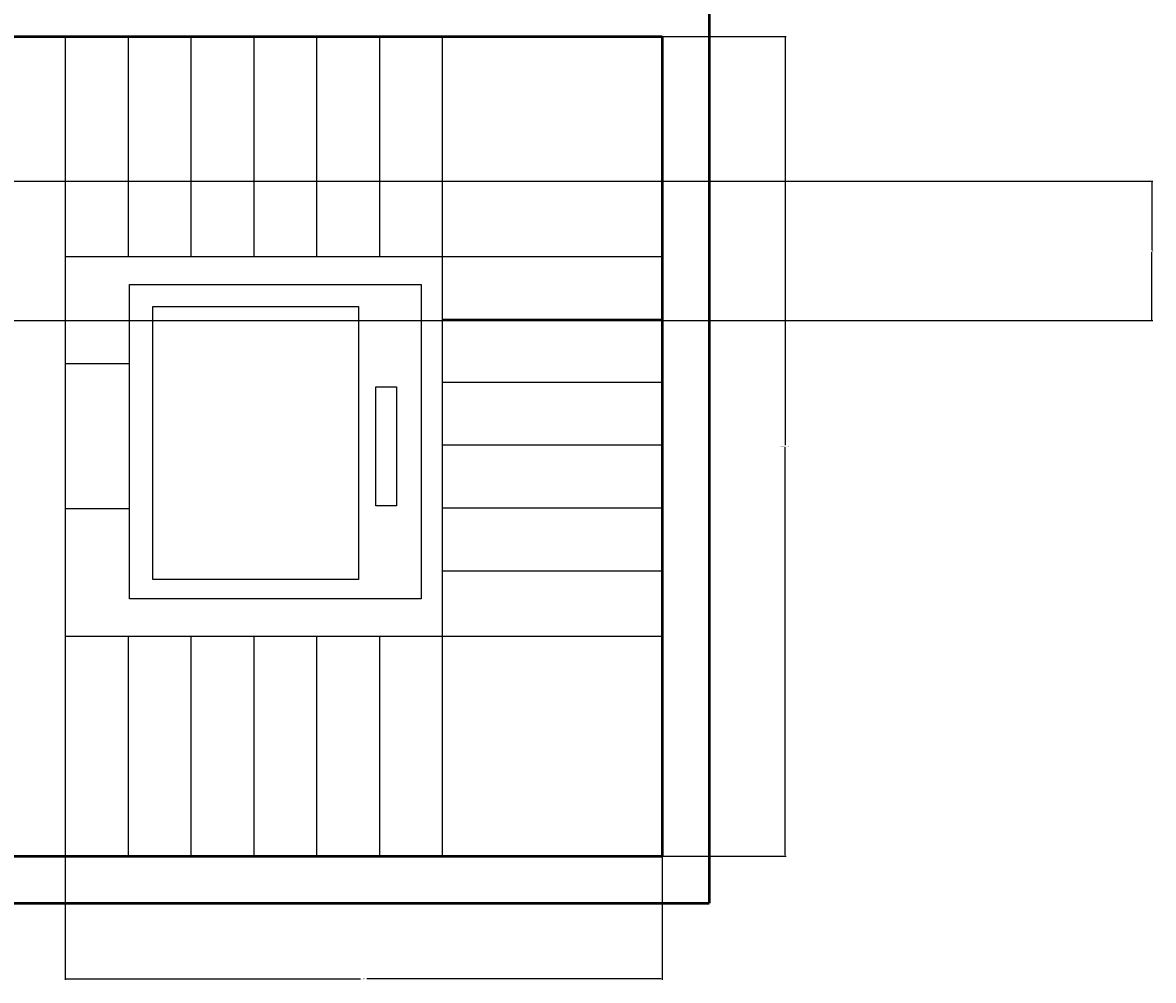
# Model space of a CAD drawing. Units: inches. Extents: x 7359 to 7979, y 33027 to 34263.
# Tile 30 of 32: x 7753 to 7969, y 33750 to 33933. Entities that reach past the tile are written whole.
import ezdxf

# ---------------------------------------------------------------- set-up
doc = ezdxf.new("R2010")
doc.units = ezdxf.units.IN
for name, color, linetype, lineweight in [('A-ANNO-DIMS', 2, 'Continuous', 18), ('A-CONV', 6, 'Continuous', 25), ('A-FLOR-STRS', 7, 'Continuous', 25), ('A-WALL', 7, 'Continuous', 50)]:
    doc.layers.add(name, color=color, linetype=linetype, lineweight=lineweight)
doc.styles.get("Standard").update_dxf_attribs({"font": 'arial.ttf'})
doc.dimstyles.get("Standard").update_dxf_attribs({"dimtxt": 0.18, "dimasz": 0.18, "dimexe": 0.18, "dimexo": 0.0625, "dimgap": 0.09, "dimtad": 0, "dimtih": 1, "dimtoh": 1, "dimdec": 4, "dimzin": 0, "dimdsep": 46, "dimtxsty": 'Standard', "dimcen": 0.09, "dimadec": 0, "dimazin": 0, "dimtfac": 1, "dimtdec": 4, "dimtofl": 0, "dimtmove": 0, "dimatfit": 3, "dimfxl": 1, "dimtolj": 1, "dimtzin": 0, "dimarcsym": 0})

# ---------------------------------------------------------------- blocks, each defined once
blk = doc.blocks.new('STAIR-THREE-FLIGHT')
for p, q in [((0, 156.5), (0, 114.5)), ((12, 156.5), (12, 114.5)), ((24, 156.5), (24, 114.5)), ((36, 156.5), (36, 114.5)), ((48, 156.5), (48, 114.5)), ((60, 156.5), (60, 114.5)), ((72, 156.5), (72, 0)), ((0, 114.5), (114, 114.5)), ((0, 114.5), (0, 42)), ((72, 102.5), (114, 102.5)), ((72, 90.5), (114, 90.5)), ((72, 78.5), (114, 78.5)), ((72, 66.5), (114, 66.5)), ((72, 54.5), (114, 54.5)), ((0, 42), (114, 42)), ((0, 42), (0, 0)), ((12, 42), (12, 0)), ((24, 42), (24, 0)), ((36, 42), (36, 0)), ((48, 42), (48, 0)), ((60, 42), (60, 0))]:
    blk.add_line(p, q)
blk = doc.blocks.new('LIFT-PLAN')
for p, q in [((0, 44.9), (12.25, 44.9)), ((0, 17.24), (12.25, 17.24))]:
    blk.add_line(p, q)
for points in [[(12.25, 60.03), (67.98, 60.03), (67.98, 0), (12.25, 0)], [(16.72, 55.81), (56.03, 55.81), (56.03, 3.68), (16.72, 3.68)], [(59.32, 40.45), (63.26, 40.45), (63.26, 17.73), (59.32, 17.73)]]:
    blk.add_lwpolyline(points, close=True)
blk = doc.blocks.new('*D50')
at = {"layer": 'A-ANNO-DIMS', "color": 0, "lineweight": -2, "transparency": 16777216}
for p, q in [((7875.05, 33930.33), (7898.65, 33930.33)), ((7898.47, 33930.15), (7898.47, 33852.27)), ((7898.47, 33774.01), (7898.47, 33851.9)), ((7875.05, 33773.83), (7898.65, 33773.83))]:
    blk.add_line(p, q, dxfattribs=at)
at = {"layer": 'A-ANNO-DIMS', "color": 0, "transparency": 16777216}
for points in [[(7898.44, 33930.15), (7898.5, 33930.15), (7898.47, 33930.33)], [(7898.44, 33774.01), (7898.5, 33774.01), (7898.47, 33773.83)]]:
    blk.add_solid(points, dxfattribs=at)
at = {"layer": 'Defpoints', "color": 0, "transparency": 16777216}
for p in [(7874.99, 33930.33), (7898.47, 33930.33), (7874.99, 33773.83)]:
    blk.add_point(p, dxfattribs=at)
at = {"layer": 'A-ANNO-DIMS', "color": 0, "transparency": 16777216, "insert": (7898.47, 33852.08), "char_height": 0.18, "attachment_point": 5}
blk.add_mtext('\\A1;STAIR 157 TYP.', dxfattribs=at)
blk = doc.blocks.new('*D51')
at = {"layer": 'A-ANNO-DIMS', "color": 0, "lineweight": -2, "transparency": 16777216}
for p, q in [((7760.99, 33773.77), (7760.99, 33750.18)), ((7874.99, 33773.77), (7874.99, 33750.18)), ((7761.17, 33750.36), (7817.4, 33750.36)), ((7874.81, 33750.36), (7818.58, 33750.36))]:
    blk.add_line(p, q, dxfattribs=at)
at = {"layer": 'A-ANNO-DIMS', "color": 0, "transparency": 16777216}
for points in [[(7761.17, 33750.39), (7761.17, 33750.33), (7760.99, 33750.36)], [(7874.81, 33750.39), (7874.81, 33750.33), (7874.99, 33750.36)]]:
    blk.add_solid(points, dxfattribs=at)
at = {"layer": 'Defpoints', "color": 0, "transparency": 16777216}
for p in [(7760.99, 33773.83), (7874.99, 33773.83), (7874.99, 33750.36)]:
    blk.add_point(p, dxfattribs=at)
at = {"layer": 'A-ANNO-DIMS', "color": 0, "transparency": 16777216, "insert": (7817.99, 33750.36), "char_height": 0.18, "attachment_point": 5}
blk.add_mtext('\\A1;114 TYP.', dxfattribs=at)
blk = doc.blocks.new('*D82')
at = {"layer": 'A-ANNO-DIMS', "color": 0, "lineweight": -2, "transparency": 16777216}
for p, q in [((7689.55, 33902.73), (7968.68, 33902.73)), ((7968.5, 33902.55), (7968.5, 33889.59)), ((7968.5, 33876.26), (7968.5, 33889.23)), ((7689.55, 33876.08), (7968.68, 33876.08))]:
    blk.add_line(p, q, dxfattribs=at)
at = {"layer": 'A-ANNO-DIMS', "color": 0, "transparency": 16777216}
for points in [[(7968.47, 33902.55), (7968.53, 33902.55), (7968.5, 33902.73)], [(7968.47, 33876.26), (7968.53, 33876.26), (7968.5, 33876.08)]]:
    blk.add_solid(points, dxfattribs=at)
at = {"layer": 'Defpoints', "color": 0, "transparency": 16777216}
for p in [(7689.49, 33902.73), (7968.5, 33902.73), (7689.49, 33876.08)]:
    blk.add_point(p, dxfattribs=at)
at = {"layer": 'A-ANNO-DIMS', "color": 0, "transparency": 16777216, "insert": (7968.5, 33889.41), "char_height": 0.18, "attachment_point": 5}
blk.add_mtext('\\A1;26.65', dxfattribs=at)

msp = doc.modelspace()

# ---------------------------------------------------------------- linework, layer by layer
at = {"layer": 'A-WALL'}
for p, q in [((7883.9915, 34233.3339), (7883.9915, 33764.8339)), ((7698.4915, 33930.3339), (7874.9915, 33930.3339)), ((7874.9915, 33930.3339), (7874.9915, 33773.8339)), ((7698.4915, 33773.8339), (7874.9915, 33773.8339)), ((7458.5915, 33764.8339), (7883.9915, 33764.8339))]:
    msp.add_line(p, q, dxfattribs=at)

# ---------------------------------------------------------------- block references
at = {"layer": 'A-CONV'}
msp.add_blockref('LIFT-PLAN', (7760.991, 33822.985), dxfattribs=at)
at = {"layer": 'A-FLOR-STRS'}
msp.add_blockref('STAIR-THREE-FLIGHT', (7760.991, 33773.834), dxfattribs=at)

# ---------------------------------------------------------------- dimensions: what is measured, and where the dimension line sits
at = {"layer": 'A-ANNO-DIMS'}
dim = msp.add_linear_dim(base=(7898.4664840368, 33930.3339283577), p1=(7874.9914840368, 33773.8339283577), p2=(7874.9914840368, 33930.3339283577), angle=90, text='STAIR <> TYP.', dimstyle='Standard', override={"dimdec": 0, "dimlfac": 1, "dimrnd": 0, "dimzin": 0, "dimdsep": 46, "dimlunit": 2}, dxfattribs=at)
dim.commit()
dim.dimension.update_dxf_attribs({"geometry": '*D50', "text_midpoint": (7898.4664840368, 33852.0839283577)})
dim = msp.add_linear_dim(base=(7968.502, 33902.7339), p1=(7689.4915, 33876.0839), p2=(7689.4915, 33902.7339), angle=90, dimstyle='Standard', override={"dimdec": 2, "dimlfac": 1, "dimrnd": 0, "dimzin": 0, "dimdsep": 46, "dimlunit": 2}, dxfattribs=at)
dim.commit()
dim.dimension.update_dxf_attribs({"geometry": '*D82', "text_midpoint": (7968.502, 33889.4089)})
dim = msp.add_linear_dim(base=(7874.9915, 33750.3589), p1=(7760.9915, 33773.8339), p2=(7874.9915, 33773.8339), text='<> TYP.', dimstyle='Standard', override={"dimdec": 0, "dimlfac": 1, "dimrnd": 0, "dimzin": 0, "dimdsep": 46, "dimlunit": 2}, dxfattribs=at)
dim.commit()
dim.dimension.update_dxf_attribs({"geometry": '*D51', "text_midpoint": (7817.9915, 33750.3589)})

doc.saveas('drawing.dxf')
